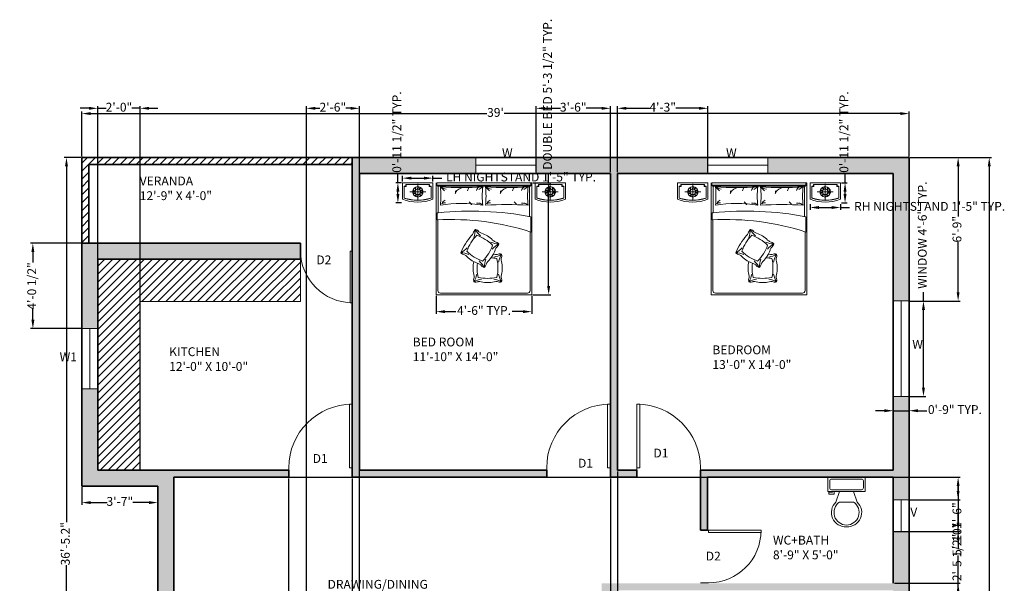
# Model space of a CAD drawing. Units: inches. Extents: x -34 to 523, y -544 to 92.
# Tile 2 of 2: x -34 to 523, y -227 to 92. Entities that reach past the tile are written whole.
import ezdxf

# ---------------------------------------------------------------- set-up
doc = ezdxf.new("R2010")
doc.units = ezdxf.units.IN
for name, color, linetype, lineweight in [('A-ANNO-DIMS', 2, 'Continuous', 18), ('A-ANNO-TEXT', 7, 'Continuous', 18), ('A-AREA-IDEN', 7, 'Continuous', 25), ('A-DOOR', 4, 'Continuous', 18), ('A-FLOR-FIXT', 9, 'Continuous', 18), ('A-GLAZ', 4, 'Continuous', 18), ('A-WALL', 7, 'Continuous', 35), ('furn', 28, 'Continuous', 18)]:
    doc.layers.add(name, color=color, linetype=linetype, lineweight=lineweight)
doc.layers.add('A-FLOR-FIXT-PATT', color=215, linetype='Continuous', lineweight=13, true_color=0xa953a0)
doc.layers.add('A-WALL-PATT', color=244, linetype='Continuous', lineweight=13, true_color=0x991b1e)
doc.styles.get("Standard").update_dxf_attribs({"font": 'arial.ttf'})
doc.dimstyles.new('ISO-25', dxfattribs={"dimtxt": 5, "dimasz": 5, "dimexe": 1.25, "dimexo": 0.625, "dimtad": 0, "dimlunit": 3, "dimtxsty": 'Standard', "dimcen": 2.5, "dimadec": 0, "dimazin": 0, "dimtfac": 1, "dimtmove": 0, "dimatfit": 3, "dimfxl": 1, "dimarcsym": 0})
pattern_1 = [(45, (-297.2655, -18.6034), (-2.245064, 2.245064), [])]

# ---------------------------------------------------------------- blocks, each defined once
blk = doc.blocks.new('*U2')
for p, q in [((0, 0), (0, -6)), ((40, 0), (40, -6))]:
    blk.add_line(p, q)
blk.add_lwpolyline([(0, 0), (0, 40), (1.75, 40), (1.75, 0)], close=True)
blk.add_arc((0, 0), 40, 0, 90)
blk = doc.blocks.new('*U4')
for p, q in [((9.5, -6), (9.5, -2)), ((-10, -8.5), (-8, -8.5)), ((-10, -9.5), (-10, -8.5)), ((-7, -9.5), (-10, -9.5)), ((-8, -8.5), (-8, -8)), ((-7, -8), (-7, -9.5)), ((-4, -8), (-6, -14)), ((4, -8), (6, -14)), ((4, -14), (-4, -14))]:
    blk.add_line(p, q)
blk.add_lwpolyline([(10.5, -8), (10.5, 0), (-10.5, 0), (-10.5, -8)], close=True)
for points in [[(-9.5, -2), (-9.5, -6)], [(8.5, -1), (-8.5, -1)], [(-8.5, -7), (8.5, -7)]]:
    blk.add_lwpolyline(points)
for centre, radius, start, end in [((-8.625, -1.875), 0.8839, 81.8699, 188.1301), ((8.625, -1.875), 0.8839, 351.8699, 98.1301), ((-8.625, -6.125), 0.8839, 171.869898, 278.1301), ((8.625, -6.125), 0.8839, 261.8699, 8.1301), ((-0.4772, -19.9188), 8.0953, 133.01722, 273.38), ((0.0374, -19.8731), 7.127, 124.50543, 269.7), ((-0.0373, -19.8731), 7.127, 270.3, 55.4946), ((0.4773, -19.9188), 8.0953, 266.62, 46.9828)]:
    blk.add_arc(centre, radius, start, end)
blk = doc.blocks.new('*D6')
at = {"layer": 'A-ANNO-DIMS', "color": 0, "lineweight": -2, "transparency": 16777216}
for p, q in [((1.12, -173.01), (1.12, -182.93)), ((44.12, -175.22), (44.12, -182.93)), ((6.12, -181.68), (15.36, -181.68)), ((39.12, -181.68), (29.89, -181.68))]:
    blk.add_line(p, q, dxfattribs=at)
at = {"layer": 'A-ANNO-DIMS', "color": 0, "transparency": 16777216}
for points in [[(6.12, -180.85), (6.12, -182.51), (1.12, -181.68)], [(39.12, -180.85), (39.12, -182.51), (44.12, -181.68)]]:
    blk.add_solid(points, dxfattribs=at)
at = {"layer": 'Defpoints', "color": 0, "transparency": 16777216}
for p in [(1.12, -172.38), (44.12, -174.6), (44.12, -181.68)]:
    blk.add_point(p, dxfattribs=at)
at = {"layer": 'A-ANNO-DIMS', "color": 0, "transparency": 16777216, "insert": (22.62, -181.68), "char_height": 5, "attachment_point": 5}
blk.add_mtext('3\'-7"', dxfattribs=at)
blk = doc.blocks.new('*D12')
at = {"layer": 'A-ANNO-DIMS', "color": 0, "lineweight": -2, "transparency": 16777216}
for p, q in [((0.5, 13.62), (-8.81, 13.62)), ((-7.56, 8.62), (-7.56, -192.86)), ((-7.56, -418.58), (-7.56, -217.1)), ((43.5, -423.58), (-8.81, -423.58))]:
    blk.add_line(p, q, dxfattribs=at)
at = {"layer": 'A-ANNO-DIMS', "color": 0, "transparency": 16777216}
for points in [[(-8.39, 8.62), (-6.73, 8.62), (-7.56, 13.62)], [(-8.39, -418.58), (-6.73, -418.58), (-7.56, -423.58)]]:
    blk.add_solid(points, dxfattribs=at)
at = {"layer": 'Defpoints', "color": 0, "transparency": 16777216}
for p in [(1.12, 13.62), (-7.56, -423.58), (44.12, -423.58)]:
    blk.add_point(p, dxfattribs=at)
at = {"layer": 'A-ANNO-DIMS', "color": 0, "transparency": 16777216, "insert": (-7.56, -204.98), "char_height": 5, "attachment_point": 5, "rotation": 90}
blk.add_mtext('36\'-5.2"', dxfattribs=at)
blk = doc.blocks.new('*D13')
at = {"layer": 'A-ANNO-DIMS', "color": 0, "lineweight": -2, "transparency": 16777216}
for p, q in [((1.12, 14.24), (1.12, 39.73)), ((469.12, 14.24), (469.12, 39.73)), ((6.12, 38.48), (230.26, 38.48)), ((464.12, 38.48), (239.99, 38.48))]:
    blk.add_line(p, q, dxfattribs=at)
at = {"layer": 'A-ANNO-DIMS', "color": 0, "transparency": 16777216}
for points in [[(6.12, 39.32), (6.12, 37.65), (1.12, 38.48)], [(464.12, 39.32), (464.12, 37.65), (469.12, 38.48)]]:
    blk.add_solid(points, dxfattribs=at)
at = {"layer": 'Defpoints', "color": 0, "transparency": 16777216}
for p in [(469.12, 38.48), (1.12, 13.62), (469.12, 13.62)]:
    blk.add_point(p, dxfattribs=at)
at = {"layer": 'A-ANNO-DIMS', "color": 0, "transparency": 16777216, "insert": (235.12, 38.48), "char_height": 5, "attachment_point": 5}
blk.add_mtext("39'", dxfattribs=at)
blk = doc.blocks.new('*D14')
at = {"layer": 'A-ANNO-DIMS', "color": 0, "lineweight": -2, "transparency": 16777216}
for p, q in [((469.75, 13.62), (515.68, 13.62)), ((514.43, 8.62), (514.43, -233.57)), ((514.43, -494.38), (514.43, -252.2)), ((469.75, -499.38), (515.68, -499.38))]:
    blk.add_line(p, q, dxfattribs=at)
at = {"layer": 'A-ANNO-DIMS', "color": 0, "transparency": 16777216}
for points in [[(513.6, 8.62), (515.26, 8.62), (514.43, 13.62)], [(513.6, -494.38), (515.26, -494.38), (514.43, -499.38)]]:
    blk.add_solid(points, dxfattribs=at)
at = {"layer": 'Defpoints', "color": 0, "transparency": 16777216}
for p in [(469.12, 13.62), (469.12, -499.38), (514.43, -499.38)]:
    blk.add_point(p, dxfattribs=at)
at = {"layer": 'A-ANNO-DIMS', "color": 0, "transparency": 16777216, "insert": (514.43, -242.88), "char_height": 5, "attachment_point": 5, "rotation": 90}
blk.add_mtext('42\'-9"', dxfattribs=at)
blk = doc.blocks.new('BED-DOUBLE')
for p, q in [((0.94, 61.53), (53.14, 61.53)), ((1.21, 61.99), (1.21, 46.38)), ((52.84, 61.99), (52.84, 44.35))]:
    blk.add_line(p, q)
for points in [[(0, 63.46), (0, 0), (54.08, 0), (54.08, 63.46)], [(53.58, 63.46), (53.58, 61.99), (0.31, 61.99), (0.31, 63.46), (54.08, 63.46)]]:
    blk.add_lwpolyline(points)
for points in [[(2.4, 50.65, 0.058596), (2.4, 61.1, 0.036889), (26.34, 61.1, 0.052163), (26.34, 50.65, 0.093111)], [(27.89, 50.65, 0.058596), (27.89, 61.1, 0.036648), (51.99, 61.1, 0.052163), (51.99, 50.65, 0.036967)], [(0.47, 46.38), (1.21, 46.38, -0.072944), (53.58, 44.2), (53.58, 35.53, 0.092568), (0.47, 42.4)]]:
    blk.add_lwpolyline(points, format="xyb", close=True)
for points in [[(0.94, 42.43), (0.94, 2.5, 0.414214), (2.5, 0.94), (51.58, 0.94, 0.414214), (53.14, 2.5), (53.14, 35.68)], [(17.36, 24.65, 0.111006), (26.29, 19.1, 0.119549), (31.92, 28.13, 0.107813), (23.02, 33.71)], [(22.97, 33.69, 0.121865), (17.36, 24.65, 0.121865)], [(21.24, 32.47, 0.091296), (22.19, 37.05, 0.091296), (25.07, 33.37, 0.091296)], [(27.19, 15.52, 0.159461), (28.4, 17.67, -0.076283), (29.36, 19, 0.115075), (33.28, 25.3, -0.076283), (34.06, 26.75, 0.159461), (35.45, 28.79)], [(30.88, 29.75, 0.091296), (35.45, 28.79, 0.091296), (31.76, 25.91, 0.091296)], [(18.5, 22.82, 0.091296), (13.92, 23.79, 0.091296), (17.61, 26.66, 0.091296)], [(32.56, 21.35, 0.091296), (36.96, 22.96, 0.091296), (35.34, 18.57, 0.091296)], [(36.96, 7.33, 0.159461), (36.85, 9.79, -0.076283), (36.96, 11.43, 0.115075), (36.96, 18.85, -0.076283), (36.85, 20.49, 0.159461), (36.96, 22.96)], [(23.79, 9.88, 0.111006), (34.31, 9.89, 0.119549), (34.31, 20.53, 0.033212), (31.08, 21.02)], [(28.14, 20.1, 0.091296), (27.19, 15.52, 0.091296), (24.3, 19.2)], [(25.72, 8.93, 0.091296), (21.33, 7.33, 0.091296), (22.94, 11.71, 0.091296)], [(35.34, 11.71, 0.091296), (36.96, 7.33, 0.091296), (32.56, 8.93)]]:
    blk.add_lwpolyline(points, format="xyb")
for centre, radius, start, end in [((0.94, 62.47), 0.938, 180, 270), ((53.14, 62.47), 0.938, 270, 0), ((7.95, 69.83), 10.35, 237.5379, 257.5233), ((-5.44, 51.33), 12.52, 36.4935, 51.2792), ((8.37, 58.13), 2.6, 335.8927, 16.1192), ((15.89, 54.9), 5.79, 96.6849, 148.3182), ((21.75, 58.2), 4.06, 141.8174, 169.8987), ((26.89, 57.62), 4.37, 130.5354, 160.3558), ((29.62, 53.94), 7.88, 114.6457, 134.1585), ((20.06, 51.33), 12.52, 36.4935, 51.2792), ((33.45, 69.83), 10.35, 237.5379, 257.5233), ((33.87, 58.13), 2.6, 335.8927, 16.1192), ((41.39, 54.9), 5.79, 96.6849, 148.3182), ((47.25, 58.2), 4.06, 141.8174, 169.8987), ((52.39, 57.62), 4.37, 130.5354, 160.3558), ((55.11, 53.94), 7.88, 114.6457, 134.1585), ((6.51, 50.41), 3.47, 114.2916, 160.9896), ((4.71, 49.68), 2.38, 76.4823, 128.5563), ((9.44, 43.38), 13.05, 36.2085, 45.0849), ((19.1, 51.09), 0.876, 353.7543, 77.2187), ((23.28, 47.66), 4.27, 44.406, 96.8342), ((24.08, 49.15), 2.71, 33.6349, 90.8456), ((32.01, 50.41), 3.47, 114.2916, 160.9896), ((30.2, 49.68), 2.38, 76.4823, 128.5563), ((34.94, 43.38), 13.05, 36.2085, 45.0849), ((44.59, 51.09), 0.876, 353.7543, 77.2187), ((48.78, 47.66), 4.27, 44.406, 96.8342), ((49.58, 49.15), 2.71, 33.6349, 90.8456), ((45.61, 10.83), 34.23, 138.3818, 157.7644), ((16.14, 37.37), 5.43, 315.5854, 333.0343), ((24.86, 34.13), 3.96, 132.4658, 168.7065), ((21.14, 33.37), 3.82, 37.2937, 74.0973), ((27.43, 40.04), 5.43, 233.2983, 250.7472), ((20.42, 19.44), 16.33, 45.1307, 71.3884), ((35.73, 34.9), 5.43, 225.7718, 243.2208), ((32.63, 26.46), 3.66, 39.4726, 79.6505), ((16.84, 26.47), 3.96, 222.6522, 258.8929), ((13.63, 17.74), 5.43, 45.7718, 63.2208), ((29.14, 7.07), 16.33, 77.0576, 78.7033), ((33.96, 28.3), 5.43, 257.6988, 275.1477), ((35.79, 19.49), 3.66, 71.3996, 111.5774), ((28.94, 33.2), 16.33, 225.1307, 251.3884), ((37.23, 15.14), 16.33, 166.8711, 193.1289), ((45.29, 15.25), 22.16, 173.1956, 194.0284), ((21.93, 12.6), 5.43, 53.2983, 70.7472), ((28.71, 19.79), 4.53, 218.7754, 250.3571), ((16.03, 10.26), 5.43, 355.0387, 12.4877), ((25.14, 8.39), 3.96, 159.3666, 195.6073), ((22.38, 11.14), 3.96, 254.5791, 290.8198), ((24.28, 2.04), 5.43, 77.6988, 95.1477), ((29.09, 23.26), 16.33, 257.0576, 283.3153), ((34.04, 2.07), 5.43, 85.2252, 102.6741), ((35.99, 11.75), 4.53, 250.7023, 282.284)]:
    blk.add_arc(centre, radius, start, end)
blk = doc.blocks.new('NIGHTSTAND-L')
for p, q in [((4.18, 5.76), (13.19, 5.76)), ((8.69, 1.26), (8.69, 10.27))]:
    blk.add_line(p, q)
blk.add_lwpolyline([(0, 1.56), (0, 10.94), (17.19, 10.94), (17.19, 1.56, -0.181818)], format="xyb", close=True)
for points in [[(1.97, 10), (1.97, 8.97), (0.94, 8.97)], [(2.06, 10), (2.06, 8.88), (0.94, 8.88)], [(1.97, 10), (15.22, 10)], [(1.97, 9.91), (15.22, 9.91)], [(15.13, 10), (15.13, 8.88), (16.26, 8.88)], [(15.22, 10), (15.22, 8.97), (16.26, 8.97)]]:
    blk.add_lwpolyline(points)
for points in [[(16.26, 8.97), (16.26, 2.22, -0.167087), (0.94, 2.22), (0.94, 8.97)], [(16.16, 8.97), (16.16, 2.28, -0.165559), (1.03, 2.28), (1.03, 8.97)]]:
    blk.add_lwpolyline(points, format="xyb")
for radius in [2.94, 1.6]:
    blk.add_circle((8.69, 5.76), radius)
for centre, radius, start, end in [((7.6, 7.7), 1.89, 208.17, 254.4897), ((7.47, 7.56), 1.44, 196.3002, 256.538), ((8.95, 7.97), 1.89, 172.17, 218.4897), ((8.76, 7.93), 1.44, 160.3002, 220.538), ((10.19, 7.4), 1.89, 136.17, 182.4897), ((10.02, 7.47), 1.44, 124.3002, 184.538), ((10.86, 6.2), 1.89, 100.17, 146.4897), ((10.77, 6.36), 1.44, 88.3002, 148.538), ((10.7, 4.83), 1.89, 64.17, 110.4897), ((10.72, 5.02), 1.44, 52.3002, 112.538), ((9.77, 3.83), 1.89, 28.17, 74.4897), ((6.65, 6.51), 1.44, 232.3002, 292.538), ((6.67, 6.69), 1.89, 244.17, 290.4897), ((6.6, 5.17), 1.44, 268.3002, 328.538), ((6.51, 5.33), 1.89, 280.17, 326.4897), ((7.35, 4.06), 1.44, 304.3002, 4.538), ((7.18, 4.13), 1.89, 316.17, 2.4897), ((8.61, 3.6), 1.44, 340.3002, 40.538), ((8.42, 3.56), 1.89, 352.17, 38.4897), ((9.9, 3.97), 1.44, 16.3002, 76.538)]:
    blk.add_arc(centre, radius, start, end)
blk = doc.blocks.new('NIGHTSTAND-R')
for p, q in [((13.02, 5.76), (4, 5.76)), ((8.51, 1.25), (8.51, 10.27))]:
    blk.add_line(p, q)
blk.add_lwpolyline([(17.19, 1.56), (17.19, 10.94), (0, 10.94), (0, 1.56, 0.181818)], format="xyb", close=True)
for points in [[(1.97, 10), (1.97, 8.97), (0.94, 8.97)], [(2.06, 10), (2.06, 8.88), (0.94, 8.88)], [(15.22, 10), (1.97, 10)], [(15.22, 9.91), (1.97, 9.91)], [(15.13, 10), (15.13, 8.88), (16.26, 8.88)], [(15.22, 10), (15.22, 8.97), (16.26, 8.97)]]:
    blk.add_lwpolyline(points)
for points in [[(0.94, 8.97), (0.94, 2.22, 0.167087), (16.26, 2.22), (16.26, 8.97)], [(1.03, 8.97), (1.03, 2.28, 0.165559), (16.16, 2.28), (16.16, 8.97)]]:
    blk.add_lwpolyline(points, format="xyb")
for radius in [2.94, 1.6]:
    blk.add_circle((8.51, 5.76), radius)
for centre, radius, start, end in [((6.47, 5.02), 1.44, 67.462, 127.6998), ((6.49, 4.83), 1.89, 69.5103, 115.83), ((7.42, 3.82), 1.89, 105.5103, 151.83), ((6.43, 6.36), 1.44, 31.462, 91.6998), ((6.33, 6.19), 1.89, 33.5103, 79.83), ((7.17, 7.47), 1.44, 355.462, 55.6998), ((7, 7.39), 1.89, 357.5103, 43.83), ((8.43, 7.92), 1.44, 319.462, 19.6998), ((8.46, 8.05), 1.89, 321.5103, 7.83), ((9.93, 7.64), 1.44, 283.462, 343.6998), ((9.81, 7.78), 1.89, 285.5103, 331.83), ((7.3, 3.96), 1.44, 103.462, 163.6998), ((8.77, 3.55), 1.89, 141.5103, 187.83), ((8.58, 3.6), 1.44, 139.462, 199.6998), ((10.02, 4.13), 1.89, 177.5103, 223.83), ((9.84, 4.05), 1.44, 175.462, 235.6998), ((10.69, 5.33), 1.89, 213.5103, 259.83), ((10.59, 5.16), 1.44, 211.462, 271.6998), ((10.74, 6.77), 1.89, 249.5103, 295.83), ((10.76, 6.58), 1.44, 247.462, 307.6998)]:
    blk.add_arc(centre, radius, start, end)
blk = doc.blocks.new('WIN-34IN')
blk.add_line((4.5, 34), (4.5, 0))
blk.add_lwpolyline([(9, 34), (9, 0), (0, 0), (0, 34)], close=True)
blk = doc.blocks.new('WIN-54IN')
blk.add_line((4.5, 54), (4.5, 0))
blk.add_lwpolyline([(0, 54), (9, 54), (9, 0), (0, 0)], close=True)
blk = doc.blocks.new('*D22')
at = {"layer": 'A-ANNO-DIMS', "color": 0, "lineweight": -2, "transparency": 16777216}
for p, q in [((477.22, -67.6), (477.22, -62.6)), ((469.75, -67.6), (478.47, -67.6)), ((477.22, -116.6), (477.22, -72.6)), ((469.75, -121.6), (478.47, -121.6))]:
    blk.add_line(p, q, dxfattribs=at)
at = {"layer": 'A-ANNO-DIMS', "color": 0, "transparency": 16777216}
for points in [[(476.39, -72.6), (478.06, -72.6), (477.22, -67.6)], [(476.39, -116.6), (478.06, -116.6), (477.22, -121.6)]]:
    blk.add_solid(points, dxfattribs=at)
at = {"layer": 'Defpoints', "color": 0, "transparency": 16777216}
for p in [(469.12, -67.6), (477.22, -67.6), (469.12, -121.6)]:
    blk.add_point(p, dxfattribs=at)
at = {"layer": 'A-ANNO-DIMS', "color": 0, "transparency": 16777216, "insert": (477.22, -30.33), "char_height": 5, "attachment_point": 5, "rotation": 90}
blk.add_mtext('WINDOW 4\'-6" TYP.', dxfattribs=at)
blk = doc.blocks.new('*D23')
at = {"layer": 'A-ANNO-DIMS', "color": 0, "lineweight": -2, "transparency": 16777216}
for p, q in [((460.12, -122.22), (460.12, -130.95)), ((469.12, -122.22), (469.12, -130.95)), ((455.12, -129.7), (450.12, -129.7)), ((460.12, -129.7), (469.12, -129.7)), ((474.12, -129.7), (479.12, -129.7))]:
    blk.add_line(p, q, dxfattribs=at)
at = {"layer": 'A-ANNO-DIMS', "color": 0, "transparency": 16777216}
for points in [[(455.12, -128.86), (455.12, -130.53), (460.12, -129.7)], [(474.12, -128.86), (474.12, -130.53), (469.12, -129.7)]]:
    blk.add_solid(points, dxfattribs=at)
at = {"layer": 'Defpoints', "color": 0, "transparency": 16777216}
for p in [(460.12, -121.6), (469.12, -121.6), (469.12, -129.7)]:
    blk.add_point(p, dxfattribs=at)
at = {"layer": 'A-ANNO-DIMS', "color": 0, "transparency": 16777216, "insert": (494.99, -129.7), "char_height": 5, "attachment_point": 5}
blk.add_mtext('0\'-9" TYP.', dxfattribs=at)
blk = doc.blocks.new('*D24')
at = {"layer": 'A-ANNO-DIMS', "color": 0, "lineweight": -2, "transparency": 16777216}
for p, q in [((265.17, -0.64), (265.17, 4.36)), ((256.28, -0.64), (266.42, -0.64)), ((265.17, -59.1), (265.17, -5.64)), ((256.28, -64.1), (266.42, -64.1))]:
    blk.add_line(p, q, dxfattribs=at)
at = {"layer": 'A-ANNO-DIMS', "color": 0, "transparency": 16777216}
for points in [[(264.34, -5.64), (266.01, -5.64), (265.17, -0.64)], [(264.34, -59.1), (266.01, -59.1), (265.17, -64.1)]]:
    blk.add_solid(points, dxfattribs=at)
at = {"layer": 'Defpoints', "color": 0, "transparency": 16777216}
for p in [(255.65, -0.64), (265.17, -0.64), (255.65, -64.1)]:
    blk.add_point(p, dxfattribs=at)
at = {"layer": 'A-ANNO-DIMS', "color": 0, "transparency": 16777216, "insert": (265.17, 49.41), "char_height": 5, "attachment_point": 5, "rotation": 90}
blk.add_mtext('DOUBLE BED 5\'-3 1/2" TYP.', dxfattribs=at)
blk = doc.blocks.new('*D25')
at = {"layer": 'A-ANNO-DIMS', "color": 0, "lineweight": -2, "transparency": 16777216}
for p, q in [((201.57, -64.73), (201.57, -74.87)), ((255.65, -64.73), (255.65, -74.87)), ((206.57, -73.62), (212.65, -73.62)), ((250.65, -73.62), (244.58, -73.62))]:
    blk.add_line(p, q, dxfattribs=at)
at = {"layer": 'A-ANNO-DIMS', "color": 0, "transparency": 16777216}
for points in [[(206.57, -72.79), (206.57, -74.45), (201.57, -73.62)], [(250.65, -72.79), (250.65, -74.45), (255.65, -73.62)]]:
    blk.add_solid(points, dxfattribs=at)
at = {"layer": 'Defpoints', "color": 0, "transparency": 16777216}
for p in [(201.57, -64.1), (255.65, -64.1), (255.65, -73.62)]:
    blk.add_point(p, dxfattribs=at)
at = {"layer": 'A-ANNO-DIMS', "color": 0, "transparency": 16777216, "insert": (228.61, -73.62), "char_height": 5, "attachment_point": 5}
blk.add_mtext('4\'-6" TYP.', dxfattribs=at)
blk = doc.blocks.new('*D26')
at = {"layer": 'A-ANNO-DIMS', "color": 0, "lineweight": -2, "transparency": 16777216}
for p, q in [((182.5, -0.02), (182.5, 3.18)), ((187.5, 1.93), (194.7, 1.93)), ((199.7, -0.02), (199.7, 3.18)), ((199.7, 1.93), (204.7, 1.93))]:
    blk.add_line(p, q, dxfattribs=at)
at = {"layer": 'A-ANNO-DIMS', "color": 0, "transparency": 16777216}
for points in [[(187.5, 2.77), (187.5, 1.1), (182.5, 1.93)], [(194.7, 2.77), (194.7, 1.1), (199.7, 1.93)]]:
    blk.add_solid(points, dxfattribs=at)
at = {"layer": 'Defpoints', "color": 0, "transparency": 16777216}
for p in [(199.7, 1.93), (182.5, -0.64), (199.7, -0.64)]:
    blk.add_point(p, dxfattribs=at)
at = {"layer": 'A-ANNO-DIMS', "color": 0, "transparency": 16777216, "insert": (249.56, 1.93), "char_height": 5, "attachment_point": 5}
blk.add_mtext('LH NIGHTSTAND 1\'-5" TYP.', dxfattribs=at)
blk = doc.blocks.new('*D27')
at = {"layer": 'A-ANNO-DIMS', "color": 0, "lineweight": -2, "transparency": 16777216}
for p, q in [((179.92, -0.64), (179.92, 4.36)), ((181.88, -0.64), (178.67, -0.64)), ((179.92, -7.11), (179.92, -5.64)), ((181.88, -12.11), (178.67, -12.11))]:
    blk.add_line(p, q, dxfattribs=at)
at = {"layer": 'A-ANNO-DIMS', "color": 0, "transparency": 16777216}
for points in [[(179.09, -5.64), (180.76, -5.64), (179.92, -0.64)], [(179.09, -7.11), (180.76, -7.11), (179.92, -12.11)]]:
    blk.add_solid(points, dxfattribs=at)
at = {"layer": 'Defpoints', "color": 0, "transparency": 16777216}
for p in [(179.92, -0.64), (182.5, -0.64), (182.5, -12.11)]:
    blk.add_point(p, dxfattribs=at)
at = {"layer": 'A-ANNO-DIMS', "color": 0, "transparency": 16777216, "insert": (179.92, 27.99), "char_height": 5, "attachment_point": 5, "rotation": 90}
blk.add_mtext('0\'-11 1/2" TYP.', dxfattribs=at)
blk = doc.blocks.new('*D28')
at = {"layer": 'A-ANNO-DIMS', "color": 0, "lineweight": -2, "transparency": 16777216}
for p, q in [((413.1, -12.73), (413.1, -15.93)), ((418.1, -14.68), (425.29, -14.68)), ((430.29, -12.73), (430.29, -15.93)), ((430.29, -14.68), (435.29, -14.68))]:
    blk.add_line(p, q, dxfattribs=at)
at = {"layer": 'A-ANNO-DIMS', "color": 0, "transparency": 16777216}
for points in [[(418.1, -13.85), (418.1, -15.52), (413.1, -14.68)], [(425.29, -13.85), (425.29, -15.52), (430.29, -14.68)]]:
    blk.add_solid(points, dxfattribs=at)
at = {"layer": 'Defpoints', "color": 0, "transparency": 16777216}
for p in [(413.1, -12.1), (430.29, -12.1), (430.29, -14.68)]:
    blk.add_point(p, dxfattribs=at)
at = {"layer": 'A-ANNO-DIMS', "color": 0, "transparency": 16777216, "insert": (480.71, -14.68), "char_height": 5, "attachment_point": 5}
blk.add_mtext('RH NIGHTSTAND 1\'-5" TYP.', dxfattribs=at)
blk = doc.blocks.new('*D29')
at = {"layer": 'A-ANNO-DIMS', "color": 0, "lineweight": -2, "transparency": 16777216}
for p, q in [((432.87, -0.64), (432.87, 4.36)), ((430.92, -0.64), (434.12, -0.64)), ((432.87, -7.1), (432.87, -5.64)), ((430.92, -12.1), (434.12, -12.1))]:
    blk.add_line(p, q, dxfattribs=at)
at = {"layer": 'A-ANNO-DIMS', "color": 0, "transparency": 16777216}
for points in [[(432.04, -5.64), (433.7, -5.64), (432.87, -0.64)], [(432.04, -7.1), (433.7, -7.1), (432.87, -12.1)]]:
    blk.add_solid(points, dxfattribs=at)
at = {"layer": 'Defpoints', "color": 0, "transparency": 16777216}
for p in [(430.29, -0.64), (432.87, -0.64), (430.29, -12.1)]:
    blk.add_point(p, dxfattribs=at)
at = {"layer": 'A-ANNO-DIMS', "color": 0, "transparency": 16777216, "insert": (432.87, 27.99), "char_height": 5, "attachment_point": 5, "rotation": 90}
blk.add_mtext('0\'-11 1/2" TYP.', dxfattribs=at)
blk = doc.blocks.new('*D32')
at = {"layer": 'A-ANNO-DIMS', "color": 0, "lineweight": -2, "transparency": 16777216}
for p, q in [((118.12, -168.01), (118.12, -537.33)), ((154.12, -168.01), (154.12, -537.33)), ((123.12, -536.08), (128.86, -536.08)), ((149.12, -536.08), (143.39, -536.08))]:
    blk.add_line(p, q, dxfattribs=at)
at = {"layer": 'A-ANNO-DIMS', "color": 0, "transparency": 16777216}
for points in [[(123.12, -535.25), (123.12, -536.92), (118.12, -536.08)], [(149.12, -535.25), (149.12, -536.92), (154.12, -536.08)]]:
    blk.add_solid(points, dxfattribs=at)
at = {"layer": 'Defpoints', "color": 0, "transparency": 16777216}
for p in [(118.12, -167.38), (154.12, -167.38), (154.12, -536.08)]:
    blk.add_point(p, dxfattribs=at)
at = {"layer": 'A-ANNO-DIMS', "color": 0, "transparency": 16777216, "insert": (136.12, -536.08), "char_height": 5, "attachment_point": 5}
blk.add_mtext('3\'-0"', dxfattribs=at)
blk = doc.blocks.new('*D33')
at = {"layer": 'A-ANNO-DIMS', "color": 0, "lineweight": -2, "transparency": 16777216}
for p, q in [((128.12, -330.95), (128.12, 42.7)), ((133.12, 41.45), (135.81, 41.45)), ((153.12, 41.45), (150.44, 41.45)), ((158.12, -330.76), (158.12, 42.7))]:
    blk.add_line(p, q, dxfattribs=at)
at = {"layer": 'A-ANNO-DIMS', "color": 0, "transparency": 16777216}
for points in [[(133.12, 42.29), (133.12, 40.62), (128.12, 41.45)], [(153.12, 42.29), (153.12, 40.62), (158.12, 41.45)]]:
    blk.add_solid(points, dxfattribs=at)
at = {"layer": 'Defpoints', "color": 0, "transparency": 16777216}
for p in [(158.12, 41.45), (128.12, -331.58), (158.12, -331.38)]:
    blk.add_point(p, dxfattribs=at)
at = {"layer": 'A-ANNO-DIMS', "color": 0, "transparency": 16777216, "insert": (143.12, 41.45), "char_height": 5, "attachment_point": 5}
blk.add_mtext('2\'-6"', dxfattribs=at)
blk = doc.blocks.new('*D35')
at = {"layer": 'A-ANNO-DIMS', "color": 0, "lineweight": -2, "transparency": 16777216}
for p, q in [((496.82, -175.05), (496.82, -170.05)), ((469.75, -180.05), (498.07, -180.05)), ((496.82, -180.05), (496.82, -182.02)), ((469.75, -198.05), (498.07, -198.05)), ((496.82, -198.05), (496.82, -196.09)), ((496.82, -203.05), (496.82, -208.05))]:
    blk.add_line(p, q, dxfattribs=at)
at = {"layer": 'A-ANNO-DIMS', "color": 0, "transparency": 16777216}
for points in [[(495.99, -175.05), (497.66, -175.05), (496.82, -180.05)], [(495.99, -203.05), (497.66, -203.05), (496.82, -198.05)]]:
    blk.add_solid(points, dxfattribs=at)
at = {"layer": 'Defpoints', "color": 0, "transparency": 16777216}
for p in [(469.12, -180.05), (469.12, -198.05), (496.82, -198.05)]:
    blk.add_point(p, dxfattribs=at)
at = {"layer": 'A-ANNO-DIMS', "color": 0, "transparency": 16777216, "insert": (496.82, -189.05), "char_height": 5, "attachment_point": 5, "rotation": 90}
blk.add_mtext('1\'-6"', dxfattribs=at)
blk = doc.blocks.new('*D36')
at = {"layer": 'A-ANNO-DIMS', "color": 0, "lineweight": -2, "transparency": 16777216}
for p, q in [((5.12, 41.45), (0.12, 41.45)), ((10.12, -162.76), (10.12, 42.7)), ((10.12, 41.45), (14.81, 41.45)), ((34.12, 41.45), (29.44, 41.45)), ((34.12, -162.76), (34.12, 42.7)), ((39.12, 41.45), (44.12, 41.45))]:
    blk.add_line(p, q, dxfattribs=at)
at = {"layer": 'A-ANNO-DIMS', "color": 0, "transparency": 16777216}
for points in [[(5.12, 42.29), (5.12, 40.62), (10.12, 41.45)], [(39.12, 42.29), (39.12, 40.62), (34.12, 41.45)]]:
    blk.add_solid(points, dxfattribs=at)
at = {"layer": 'Defpoints', "color": 0, "transparency": 16777216}
for p in [(34.12, 41.45), (10.12, -163.38), (34.12, -163.38)]:
    blk.add_point(p, dxfattribs=at)
at = {"layer": 'A-ANNO-DIMS', "color": 0, "transparency": 16777216, "insert": (22.12, 41.45), "char_height": 5, "attachment_point": 5}
blk.add_mtext('2\'-0"', dxfattribs=at)
blk = doc.blocks.new('*D37')
at = {"layer": 'A-ANNO-DIMS', "color": 0, "lineweight": -2, "transparency": 16777216}
for p, q in [((304.12, -164.01), (304.12, -537.33)), ((300.12, -168.01), (300.12, -537.33)), ((295.12, -536.08), (290.12, -536.08)), ((300.12, -536.08), (304.12, -536.08)), ((309.12, -536.08), (314.12, -536.08))]:
    blk.add_line(p, q, dxfattribs=at)
at = {"layer": 'A-ANNO-DIMS', "color": 0, "transparency": 16777216}
for points in [[(295.12, -535.25), (295.12, -536.92), (300.12, -536.08)], [(309.12, -535.25), (309.12, -536.92), (304.12, -536.08)]]:
    blk.add_solid(points, dxfattribs=at)
at = {"layer": 'Defpoints', "color": 0, "transparency": 16777216}
for p in [(304.12, -163.38), (300.12, -167.38), (304.12, -536.08)]:
    blk.add_point(p, dxfattribs=at)
at = {"layer": 'A-ANNO-DIMS', "color": 0, "transparency": 16777216, "insert": (321.4, -536.08), "char_height": 5, "attachment_point": 5}
blk.add_mtext('0\'-4"', dxfattribs=at)
blk = doc.blocks.new('*D38')
at = {"layer": 'A-ANNO-DIMS', "color": 0, "lineweight": -2, "transparency": 16777216}
for p, q in [((258.09, 5.38), (258.09, 42.7)), ((263.09, 41.45), (271.84, 41.45)), ((295.12, 41.45), (286.37, 41.45)), ((300.12, 5.24), (300.12, 42.7))]:
    blk.add_line(p, q, dxfattribs=at)
at = {"layer": 'A-ANNO-DIMS', "color": 0, "transparency": 16777216}
for points in [[(263.09, 42.29), (263.09, 40.62), (258.09, 41.45)], [(295.12, 42.29), (295.12, 40.62), (300.12, 41.45)]]:
    blk.add_solid(points, dxfattribs=at)
at = {"layer": 'Defpoints', "color": 0, "transparency": 16777216}
for p in [(300.12, 41.45), (258.09, 4.75), (300.12, 4.62)]:
    blk.add_point(p, dxfattribs=at)
at = {"layer": 'A-ANNO-DIMS', "color": 0, "transparency": 16777216, "insert": (279.1, 41.45), "char_height": 5, "attachment_point": 5}
blk.add_mtext('3\'-6"', dxfattribs=at)
blk = doc.blocks.new('*D39')
at = {"layer": 'A-ANNO-DIMS', "color": 0, "lineweight": -2, "transparency": 16777216}
for p, q in [((304.12, 5.24), (304.12, 42.7)), ((309.12, 41.45), (322.33, 41.45)), ((350.27, 41.45), (337.07, 41.45)), ((355.27, 5.38), (355.27, 42.7))]:
    blk.add_line(p, q, dxfattribs=at)
at = {"layer": 'A-ANNO-DIMS', "color": 0, "transparency": 16777216}
for points in [[(309.12, 42.29), (309.12, 40.62), (304.12, 41.45)], [(350.27, 42.29), (350.27, 40.62), (355.27, 41.45)]]:
    blk.add_solid(points, dxfattribs=at)
at = {"layer": 'Defpoints', "color": 0, "transparency": 16777216}
for p in [(355.27, 41.45), (304.12, 4.62), (355.27, 4.75)]:
    blk.add_point(p, dxfattribs=at)
at = {"layer": 'A-ANNO-DIMS', "color": 0, "transparency": 16777216, "insert": (329.7, 41.45), "char_height": 5, "attachment_point": 5}
blk.add_mtext('4\'-3"', dxfattribs=at)
blk = doc.blocks.new('*D40')
at = {"layer": 'A-ANNO-DIMS', "color": 0, "lineweight": -2, "transparency": 16777216}
for p, q in [((0.5, -34.92), (-27.83, -34.92)), ((-26.58, -39.92), (-26.58, -45.88)), ((-26.58, -78.24), (-26.58, -72.28)), ((0.59, -83.24), (-27.83, -83.24))]:
    blk.add_line(p, q, dxfattribs=at)
at = {"layer": 'A-ANNO-DIMS', "color": 0, "transparency": 16777216}
for points in [[(-27.41, -39.92), (-25.74, -39.92), (-26.58, -34.92)], [(-27.41, -78.24), (-25.74, -78.24), (-26.58, -83.24)]]:
    blk.add_solid(points, dxfattribs=at)
at = {"layer": 'Defpoints', "color": 0, "transparency": 16777216}
for p in [(1.12, -34.92), (-26.58, -83.24), (1.22, -83.24)]:
    blk.add_point(p, dxfattribs=at)
at = {"layer": 'A-ANNO-DIMS', "color": 0, "transparency": 16777216, "insert": (-26.58, -59.08), "char_height": 5, "attachment_point": 5, "rotation": 90}
blk.add_mtext('4\'-0 1/2"', dxfattribs=at)
blk = doc.blocks.new('*D41')
at = {"layer": 'A-ANNO-DIMS', "color": 0, "lineweight": -2, "transparency": 16777216}
for p, q in [((53.75, -167.38), (498.07, -167.38)), ((496.82, -172.38), (496.82, -193.25)), ((496.82, -232.53), (496.82, -211.67)), ((53.78, -237.53), (498.07, -237.53))]:
    blk.add_line(p, q, dxfattribs=at)
at = {"layer": 'A-ANNO-DIMS', "color": 0, "transparency": 16777216}
for points in [[(495.99, -172.38), (497.66, -172.38), (496.82, -167.38)], [(495.99, -232.53), (497.66, -232.53), (496.82, -237.53)]]:
    blk.add_solid(points, dxfattribs=at)
at = {"layer": 'Defpoints', "color": 0, "transparency": 16777216}
for p in [(53.12, -167.38), (53.16, -237.53), (496.82, -237.53)]:
    blk.add_point(p, dxfattribs=at)
at = {"layer": 'A-ANNO-DIMS', "color": 0, "transparency": 16777216, "insert": (496.82, -202.46), "char_height": 5, "attachment_point": 5, "rotation": 90}
blk.add_mtext('5\'-10"', dxfattribs=at)
blk = doc.blocks.new('*D43')
at = {"layer": 'A-ANNO-DIMS', "color": 0, "lineweight": -2, "transparency": 16777216}
for p, q in [((469.75, 13.62), (498.07, 13.62)), ((496.82, 8.62), (496.82, -19.7)), ((496.82, -62.6), (496.82, -34.27)), ((469.75, -67.6), (498.07, -67.6))]:
    blk.add_line(p, q, dxfattribs=at)
at = {"layer": 'A-ANNO-DIMS', "color": 0, "transparency": 16777216}
for points in [[(495.99, 8.62), (497.66, 8.62), (496.82, 13.62)], [(495.99, -62.6), (497.66, -62.6), (496.82, -67.6)]]:
    blk.add_solid(points, dxfattribs=at)
at = {"layer": 'Defpoints', "color": 0, "transparency": 16777216}
for p in [(469.12, 13.62), (469.12, -67.6), (496.82, -67.6)]:
    blk.add_point(p, dxfattribs=at)
at = {"layer": 'A-ANNO-DIMS', "color": 0, "transparency": 16777216, "insert": (496.82, -26.99), "char_height": 5, "attachment_point": 5, "rotation": 90}
blk.add_mtext('6\'-9"', dxfattribs=at)
blk = doc.blocks.new('*D48')
at = {"layer": 'A-ANNO-DIMS', "color": 0, "lineweight": -2, "transparency": 16777216}
for p, q in [((496.82, -193.05), (496.82, -188.05)), ((460.75, -198.05), (498.07, -198.05)), ((496.82, -198.05), (496.82, -199.58)), ((460.75, -227.38), (498.07, -227.38)), ((496.82, -227.38), (496.82, -225.86)), ((496.82, -232.38), (496.82, -237.38))]:
    blk.add_line(p, q, dxfattribs=at)
at = {"layer": 'A-ANNO-DIMS', "color": 0, "transparency": 16777216}
for points in [[(495.99, -193.05), (497.66, -193.05), (496.82, -198.05)], [(495.99, -232.38), (497.66, -232.38), (496.82, -227.38)]]:
    blk.add_solid(points, dxfattribs=at)
at = {"layer": 'Defpoints', "color": 0, "transparency": 16777216}
for p in [(460.12, -198.05), (460.12, -227.38), (496.82, -227.38)]:
    blk.add_point(p, dxfattribs=at)
at = {"layer": 'A-ANNO-DIMS', "color": 0, "transparency": 16777216, "insert": (496.82, -212.72), "char_height": 5, "attachment_point": 5, "rotation": 90}
blk.add_mtext('2\'-5 1/2"', dxfattribs=at)

msp = doc.modelspace()

# ---------------------------------------------------------------- hatches: boundary and pattern name
at = {"layer": 'A-FLOR-FIXT-PATT'}
h = msp.add_hatch(dxfattribs=at)
h.set_pattern_fill('ANSI31', color=256)
h.set_pattern_definition(pattern_1)
h.paths.add_polyline_path([(34.124, -67.915), (124.749, -67.915), (124.749, -43.915), (10.124, -43.915), (10.124, -83.244), (10.217, -83.244), (10.217, -117.244), (10.124, -163.382), (34.124, -163.382)])
at = {"layer": 'A-WALL-PATT'}
h = msp.add_hatch(dxfattribs=at)
h.set_pattern_fill('ANSI31', color=256)
h.set_pattern_definition(pattern_1)
h.paths.add_polyline_path([(154.124, 13.618), (1.124, 13.618), (1.124, -34.915), (5.124, -34.915), (5.124, 9.618), (154.124, 9.618)])
h = msp.add_hatch(color=256, dxfattribs=at)
h.dxf.hatch_style = 1
h.paths.add_polyline_path([(10.124, -43.915), (124.749, -43.915), (124.749, -34.915), (1.124, -34.915), (1.124, -83.244), (10.124, -83.244)])
h.paths.add_polyline_path([(10.124, -117.244), (1.124, -117.244), (1.124, -172.382), (10.124, -172.382), (44.124, -172.382), (44.124, -237.534), (53.124, -237.534), (53.124, -172.382), (53.124, -167.382), (118.124, -167.382), (118.124, -163.382), (10.124, -163.382)])
h.paths.add_polyline_path([(264.093, -163.382), (158.124, -163.382), (158.124, 4.618), (224.085, 4.618), (224.085, 13.618), (158.124, 13.618), (154.124, 13.618), (154.124, -34.915), (154.124, -39.302), (154.124, -68.549), (154.124, -167.382), (264.093, -167.382)])
h.paths.add_polyline_path([(304.124, 4.618), (355.273, 4.618), (355.273, 13.618), (258.085, 13.618), (258.085, 4.618), (300.124, 4.618), (300.124, -167.382), (304.124, -167.382), (315.124, -167.382), (315.124, -163.382), (304.124, -163.382)])
h.paths.add_polyline_path([(469.124, 13.618), (389.273, 13.618), (389.273, 4.618), (460.124, 4.618), (460.124, -67.595), (469.124, -67.595)])
h.paths.add_polyline_path([(469.124, -121.595), (460.124, -121.595), (460.124, -163.382), (351.124, -163.382), (351.124, -167.382), (351.124, -197.382), (355.124, -197.382), (355.124, -167.382), (460.124, -167.382), (460.124, -180.053), (469.124, -180.053)])
h.paths.add_polyline_path([(469.124, -198.053), (460.124, -198.053), (460.124, -227.382), (295.124, -227.382), (295.124, -231.382), (295.124, -235.382), (300.506, -235.382), (304.124, -235.382), (304.124, -231.382), (460.124, -231.382), (460.124, -263.203), (469.124, -263.203)])
h.paths.add_polyline_path([(469.124, -317.203), (460.124, -317.203), (460.124, -399.382), (300.124, -399.382), (300.124, -403.382), (460.124, -403.382), (460.124, -490.382), (454.486, -490.382), (454.486, -499.382), (469.124, -499.382)])

# ---------------------------------------------------------------- linework, layer by layer
at = {"layer": 'A-FLOR-FIXT'}
for p, q in [((124.749, -43.915), (124.749, -67.915)), ((124.749, -67.915), (34.124, -67.915)), ((34.124, -163.382), (34.124, -67.915))]:
    msp.add_line(p, q, dxfattribs=at)
at = {"layer": 'A-GLAZ'}
for p, q in [((460.124, -180.053), (469.124, -180.053)), ((464.624, -198.053), (464.624, -180.053)), ((460.124, -198.053), (469.124, -198.053))]:
    msp.add_line(p, q, dxfattribs=at)
at = {"layer": 'A-WALL'}
for p, q in [((1.124, 13.618), (158.124, 13.618)), ((1.124, -34.915), (1.124, 13.618)), ((154.124, -34.915), (154.124, 13.618)), ((158.124, 13.618), (469.124, 13.618)), ((469.124, 13.618), (469.124, -499.382)), ((5.124, 9.618), (154.124, 9.618)), ((5.124, -34.915), (5.124, 9.618)), ((158.124, 4.618), (158.124, -163.382)), ((158.124, 4.618), (300.124, 4.618)), ((300.124, 4.618), (300.124, -167.382)), ((304.124, 4.618), (304.124, -163.382)), ((304.124, 4.618), (460.124, 4.618)), ((460.124, 4.618), (460.124, -163.382)), ((1.124, -172.382), (1.124, -34.915)), ((1.124, -34.915), (124.749, -34.915)), ((124.749, -34.915), (124.749, -43.915)), ((154.124, -34.915), (154.124, -167.382)), ((10.124, -163.382), (10.124, -43.915)), ((10.124, -43.915), (124.749, -43.915)), ((10.124, -163.382), (118.124, -163.382)), ((118.124, -167.382), (118.124, -163.382)), ((158.124, -163.382), (264.124, -163.382)), ((264.124, -163.382), (264.124, -167.382)), ((304.124, -163.382), (315.124, -163.382)), ((315.124, -167.382), (315.124, -163.382)), ((351.124, -167.382), (351.124, -163.382)), ((351.124, -163.382), (460.124, -163.382)), ((10.124, -172.382), (1.124, -172.382)), ((10.124, -172.382), (44.124, -172.382)), ((44.124, -172.382), (44.124, -423.58)), ((53.124, -172.382), (53.124, -167.382)), ((53.124, -167.382), (118.124, -167.382)), ((53.124, -172.382), (53.124, -331.58)), ((154.124, -167.382), (264.124, -167.382)), ((300.124, -167.382), (304.124, -167.382)), ((304.124, -167.382), (315.124, -167.382)), ((351.124, -197.382), (351.124, -167.382)), ((355.124, -197.382), (355.124, -167.382)), ((355.124, -167.382), (460.124, -167.382)), ((460.124, -167.382), (460.124, -227.382)), ((355.124, -197.382), (351.124, -197.382))]:
    msp.add_line(p, q, dxfattribs=at)

# ---------------------------------------------------------------- block references
at = {"layer": 'A-DOOR'}
for p, xscale, yscale, zscale, rotation in [((154.124, -39.302), 0.7311781832305309, 0.7311781832305309, 0.7311781832305309, 180), ((355.588, -197.382), 0.7439150042622787, 0.7439150042622787, 0.7439150042622787, 270)]:
    msp.add_blockref('*U2', p, dxfattribs=dict(at, xscale=xscale, yscale=yscale, zscale=zscale, rotation=rotation))
for p, xscale, yscale, zscale in [((154.124, -161.989), -0.8987776544859444, 0.8987776544859444, 0.8987776544859444), ((300.124, -161.977), -0.9007845201197666, 0.9007845201197666, 0.9007845201197666), ((315.124, -161.992), 0.8983245706415997, 0.8983245706415997, 0.8983245706415997)]:
    msp.add_blockref('*U2', p, dxfattribs=dict(at, xscale=xscale, yscale=yscale, zscale=zscale))
at = {"layer": 'A-FLOR-FIXT'}
msp.add_blockref('*U4', (433.708, -167.382), dxfattribs=at)
at = {"layer": 'A-GLAZ', "rotation": 89.99999999999999}
for p in [(258.085, 4.752), (389.272, 4.752)]:
    msp.add_blockref('WIN-34IN', p, dxfattribs=at)
at = {"layer": 'A-GLAZ'}
for name, p in [('WIN-54IN', (460.124, -121.595)), ('WIN-34IN', (1.216, -117.243))]:
    msp.add_blockref(name, p, dxfattribs=at)
at = {"layer": 'furn'}
for name, p in [('NIGHTSTAND-L', (182.503, -11.586)), ('BED-DOUBLE', (201.572, -64.1)), ('NIGHTSTAND-R', (257.53, -11.582)), ('NIGHTSTAND-L', (338.07, -11.586)), ('BED-DOUBLE', (357.139, -64.1)), ('NIGHTSTAND-R', (413.097, -11.582))]:
    msp.add_blockref(name, p, dxfattribs=at)

# ---------------------------------------------------------------- texts
at = {"layer": 'A-ANNO-TEXT', "char_height": 5, "attachment_point": 1}
for s, width, insert in [('{W}', 6.71404, (238.801, 18.753)), ('{W}', 6.71404, (365.559, 18.753)), ('{D2}', 15.25997, (133.774, -41.821)), ('{W}', 6.71404, (470.905, -89.595)), ('{W1}', 14.0509, (-11.431, -96.745)), ('{D1}', 11.0931, (131.72, -154.223)), ('{D1}', 11.0931, (324.463, -151.148)), ('{D1}', 11.0931, (281.821, -156.894)), ('{V}', 3.25487, (469.791, -184.569)), ('{D2}', 15.25997, (354.085, -209.467))]:
    msp.add_mtext_dynamic_manual_height_columns(s, width=width, gutter_width=12.5, heights=[0], dxfattribs=dict(at, insert=insert))
at = {"layer": 'A-AREA-IDEN', "char_height": 5, "attachment_point": 1}
for s, width, insert in [('{VERANDA\\P12\'-9" X 4\'-0"}', 69.53488, (33.867, 2.84)), ('{BED ROOM\\P11\'-10" X 14\'-0"}', 69.53972, (188.297, -88.297)), ('{KITCHEN\\P12\'-0" X 10\'-0"}', 64.46917, (50.524, -93.792)), ('{BEDROOM\\P13\'-0" X 14\'-0"}', 75.04557, (357.812, -92.74)), ('{WC+BATH\\P8\'-9" X 5\'-0"}', 51.76357, (392.079, -200.451)), ('{DRAWING/DINING\\P20\'-7" X 13\'-8"}', 144.2219, (140.129, -225.438))]:
    msp.add_mtext_dynamic_manual_height_columns(s, width=width, gutter_width=12.5, heights=[0], dxfattribs=dict(at, insert=insert))

# ---------------------------------------------------------------- dimensions: what is measured, and where the dimension line sits
at = {"layer": 'A-ANNO-DIMS'}
for base, p1, p2, text, picture, middle in [((265.173, -0.64), (255.654, -64.1), (255.654, -0.64), 'DOUBLE BED <> TYP.', '*D24', (265.173, 49.409)), ((179.924, -0.644), (182.503, -12.107), (182.503, -0.644), '<> TYP.', '*D27', (179.924, 27.987)), ((432.87, -0.641), (430.291, -12.103), (430.291, -0.641), '<> TYP.', '*D29', (432.87, 27.991)), ((477.224, -67.595), (469.124, -121.595), (469.124, -67.595), 'WINDOW <> TYP.', '*D22', (477.224, -30.335))]:
    dim = msp.add_linear_dim(base=base, p1=p1, p2=p2, angle=90, text=text, dimstyle='ISO-25', override={"dimdec": 1, "dimlfac": 1, "dimrnd": 0, "dimzin": 1, "dimdsep": 46, "dimlunit": 4, "dimfrac": 2}, dxfattribs=at)
    dim.commit()
    dim.dimension.update_dxf_attribs({"geometry": picture, "text_midpoint": middle})
for base, p1, p2, override, picture, middle in [((34.124, 41.453), (10.124, -163.382), (34.124, -163.382), {"dimdec": 1, "dimlfac": 1, "dimrnd": 0, "dimzin": 1, "dimdsep": 46, "dimlunit": 4, "dimfrac": 2}, '*D36', (22.124, 41.453)), ((158.124, 41.453), (128.124, -331.58), (158.124, -331.382), {"dimdec": 1, "dimlfac": 1, "dimrnd": 0, "dimzin": 1, "dimdsep": 46, "dimlunit": 4, "dimfrac": 2}, '*D33', (143.124, 41.453)), ((300.124, 41.453), (258.085, 4.753), (300.124, 4.618), {"dimdec": 1, "dimlfac": 1, "dimrnd": 0, "dimzin": 1, "dimdsep": 46, "dimlunit": 4, "dimfrac": 2}, '*D38', (279.105, 41.453)), ((355.273, 41.453), (304.124, 4.618), (355.273, 4.753), {"dimdec": 1, "dimlfac": 1, "dimrnd": 0, "dimzin": 1, "dimdsep": 46, "dimlunit": 4, "dimfrac": 2}, '*D39', (329.699, 41.453)), ((469.124, 38.483), (1.124, 13.618), (469.124, 13.618), {"dimclrd": 0, "dimclre": 0, "dimclrt": 0}, '*D13', (235.124, 38.483)), ((304.124, -536.082), (300.124, -167.382), (304.124, -163.382), {"dimdec": 1, "dimlfac": 1, "dimrnd": 0, "dimzin": 1, "dimdsep": 46, "dimlunit": 4, "dimfrac": 2}, '*D37', (321.395, -536.082)), ((44.124, -181.681), (1.124, -172.382), (44.124, -174.597), {"dimclrd": 0, "dimclre": 0, "dimclrt": 0}, '*D6', (22.624, -181.681)), ((154.124, -536.082), (118.124, -167.382), (154.124, -167.382), {"dimdec": 1, "dimlfac": 1, "dimrnd": 0, "dimzin": 1, "dimdsep": 46, "dimlunit": 4, "dimfrac": 2}, '*D32', (136.124, -536.082))]:
    dim = msp.add_linear_dim(base=base, p1=p1, p2=p2, dimstyle='ISO-25', override=override, dxfattribs=at)
    dim.commit()
    dim.dimension.update_dxf_attribs({"geometry": picture, "text_midpoint": middle})
for base, p1, p2, text, picture, middle in [((199.696, 1.935), (182.503, -0.644), (199.696, -0.644), 'LH NIGHTSTAND <> TYP.', '*D26', (249.556, 1.935)), ((430.291, -14.682), (413.097, -12.103), (430.291, -12.103), 'RH NIGHTSTAND <> TYP.', '*D28', (480.711, -14.682)), ((255.654, -73.619), (201.572, -64.1), (255.654, -64.1), '<> TYP.', '*D25', (228.613, -73.619)), ((469.124, -129.695), (460.124, -121.595), (469.124, -121.595), '<> TYP.', '*D23', (494.988, -129.695))]:
    dim = msp.add_linear_dim(base=base, p1=p1, p2=p2, text=text, dimstyle='ISO-25', override={"dimdec": 1, "dimlfac": 1, "dimrnd": 0, "dimzin": 1, "dimdsep": 46, "dimlunit": 4, "dimfrac": 2}, dxfattribs=at)
    dim.commit()
    dim.dimension.update_dxf_attribs({"geometry": picture, "text_midpoint": middle})
for base, p1, p2, override, picture, middle in [((-7.559, -423.58), (1.124, 13.618), (44.124, -423.58), {"dimclrd": 0, "dimclre": 0, "dimclrt": 0}, '*D12', (-7.559, -204.981)), ((514.43, -499.382), (469.124, 13.618), (469.124, -499.382), {"dimclrd": 0, "dimclre": 0, "dimclrt": 0}, '*D14', (514.43, -242.882)), ((496.824, -67.595), (469.124, 13.618), (469.124, -67.595), {"dimdec": 1, "dimlfac": 1, "dimrnd": 0, "dimzin": 1, "dimdsep": 46, "dimlunit": 4, "dimfrac": 2}, '*D43', (496.824, -26.988)), ((-26.576, -83.244), (1.124, -34.915), (1.217, -83.244), {"dimdec": 1, "dimlfac": 1, "dimrnd": 0, "dimzin": 1, "dimdsep": 46, "dimlunit": 4, "dimfrac": 2}, '*D40', (-26.576, -59.08)), ((496.824, -237.534), (53.124, -167.382), (53.155, -237.534), {"dimdec": 1, "dimlfac": 1, "dimrnd": 0, "dimzin": 1, "dimdsep": 46, "dimlunit": 4, "dimfrac": 2}, '*D41', (496.824, -202.458)), ((496.824, -198.053), (469.124, -180.053), (469.124, -198.053), {"dimdec": 1, "dimlfac": 1, "dimrnd": 0, "dimzin": 1, "dimdsep": 46, "dimlunit": 4, "dimfrac": 2}, '*D35', (496.824, -189.053)), ((496.824, -227.382), (460.124, -198.053), (460.124, -227.382), {"dimdec": 1, "dimlfac": 1, "dimrnd": 0, "dimzin": 1, "dimdsep": 46, "dimlunit": 4, "dimfrac": 2}, '*D48', (496.824, -212.718))]:
    dim = msp.add_linear_dim(base=base, p1=p1, p2=p2, angle=90, dimstyle='ISO-25', override=override, dxfattribs=at)
    dim.commit()
    dim.dimension.update_dxf_attribs({"geometry": picture, "text_midpoint": middle})

doc.saveas('drawing.dxf')
